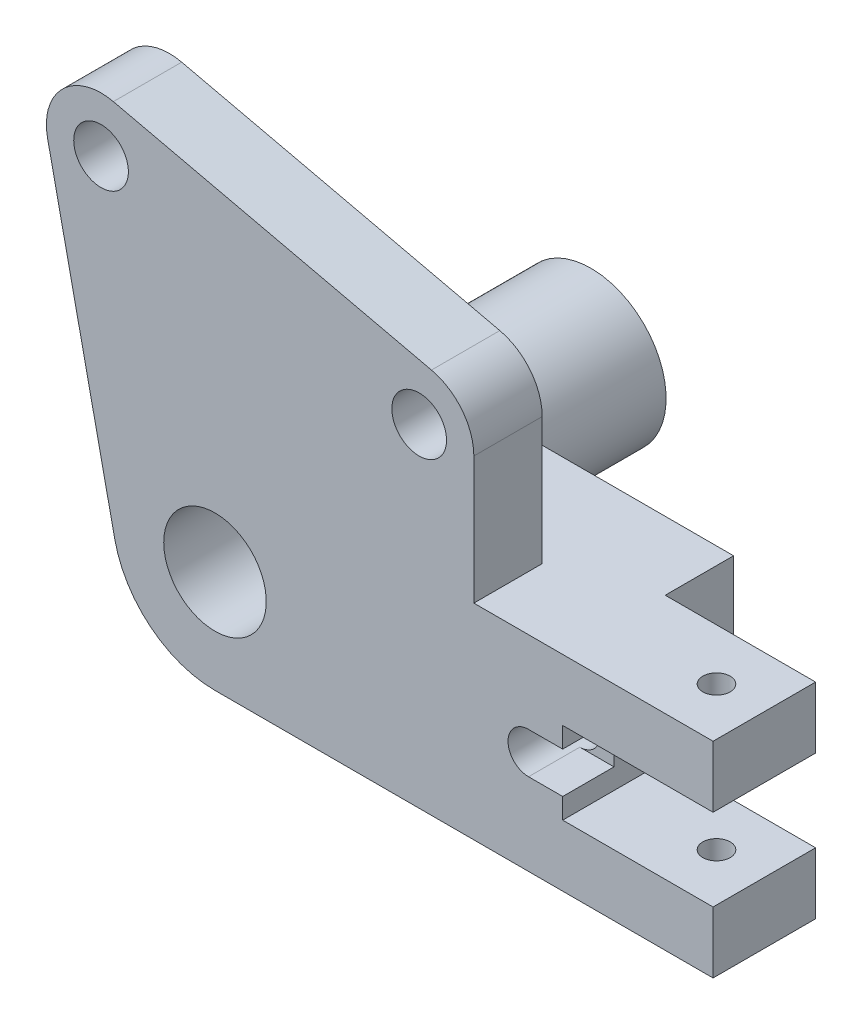
SolidWorks part; units mm, degrees
material "Plain Carbon Steel"
ref_plane "Front Plane" through (0, 0, 0) normal (0, 0, 1) x (1, 0, 0)
ref_plane "Top Plane" through (0, 0, 0) normal (0, 1, 0) x (1, 0, 0)
ref_plane "Right Plane" through (0, 0, 0) normal (1, 0, 0) x (0, 0, -1)
sketch "Bracket Plate Profile" plane through (0, 0, 0) normal (0, 0, 1) x (1, 0, 0)
  line L0 (0, 0) -> (-72.8738, 0)
  line L1 (-87.5408, 11.8571) -> (-97.3643, 57.7001)
  line L2 (-87.743, 67.1715) -> (-41.2011, 56.431)
  line L3 (-35, 48.6359) -> (-35, 30)
  line L4 (-35, 30) -> (0, 30)
  line L5 (0, 30) -> (0, 21)
  line L6 (0, 21) -> (-22, 21)
  line L7 (-22, 21) -> (-22, 9)
  line L8 (-22, 9) -> (0, 9)
  line L9 (0, 9) -> (0, 0)
  arc A0 (-35, 48.6359) -> (-41.2011, 56.431) centre (-43, 48.6359) ccw
  arc A1 (-87.743, 67.1715) -> (-97.3643, 57.7001) centre (-89.5419, 59.3763) ccw
  circle A2 centre (-89.5419, 59.3763) radius 4
  circle A3 centre (-43, 48.6359) radius 4
  arc A4 (-72.8738, 0) -> (-87.5408, 11.8571) centre (-72.8738, 15) cw
  point P13 (-35, 55)
  point P16 (-100, 70)
  point P21 (-85, 0)
  dimension "D9" = 8
  dimension "D10" = 8
  dimension "D11" = 15
  dimension "D1" = 85
  dimension "D2" = 100
  dimension "D3" = 70
  dimension "D4" = 30
  dimension "D5" = 65
  dimension "D6" = 25
  dimension "D7" = 12
  dimension "D8" = 22
extrude "Bracket Plate" add sketch "Bracket Plate Profile" along normal blind 25
sketch "Fork Slot Sketch" plane through (0, 30, 0) normal (0, 1, 0) x (1, 0, 0)
  line L0 (-35, -25) -> (-35, 0) construction
  line L1 (-35, -15) -> (-115.7544, -15)
  line L2 (-35, -15) -> (-35, 6.2579)
  line L3 (-35, 6.2579) -> (-115.7544, 6.2579)
  line L4 (-115.7544, -15) -> (-115.7544, 6.2579)
  line L5 (-41.2011, -25) -> (-87.743, -25) construction
  line L6 (0, 0) -> (-35, 0) construction
  dimension "D1" = 10
  dimension "D2" = 80.7544
  dimension "D3" = 6.2579
extrude "Fork Slot" cut sketch "Fork Slot Sketch" along normal through all
sketch "Pivot Boss Sketch" plane through (0, 0, 0) normal (0, 0, -1) x (-1, 0, 0)
  circle A0 centre (72.8738, 15) radius 11
  arc A1 (72.8738, 0) -> (87.5408, 11.8571) centre (72.8738, 15) ccw construction
  dimension "D1" = 22
extrude "Pivot Boss Ø22" add sketch "Pivot Boss Sketch" along normal blind 30
sketch "Pivot Bore Sketch" plane through (0, 0, -30) normal (0, 0, -1) x (-1, 0, 0)
  circle A0 centre (72.8738, 15) radius 7.5
  dimension "D1" = 15
extrude "Pivot Bore Ø15" cut sketch "Pivot Bore Sketch" against normal through all
sketch "Fork Notch Sketch" plane through (0, 30, 0) normal (0, 1, 0) x (1, 0, 0)
  line L0 (0, -25) -> (0, 0) construction
  line L1 (0, -10) -> (-22, -10)
  line L2 (0, -10) -> (0, 9.4983)
  line L3 (0, 9.4983) -> (-22, 9.4983)
  line L4 (-22, -10) -> (-22, 9.4983)
  line L5 (0, 0) -> (-91.4286, 0) construction
  dimension "D1" = 22
  dimension "D2" = 10
  dimension "D3" = 9.4983
extrude "Fork Notch 22x10" cut sketch "Fork Notch Sketch" against normal through all
sketch "Fork Pin Hole Sketch" plane through (0, 30, 0) normal (0, 1, 0) x (1, 0, 0)
  line L0 (0, -25) -> (0, -10) construction
  circle A0 centre (-7, -17.5) radius 2
  point P5 (0, -17.5)
  dimension "D1" = 7
  dimension "D2" = 4
extrude "Fork Pin Hole" cut sketch "Fork Pin Hole Sketch" against normal blind 30
sketch "Clamp Hole Sketch" plane through (0, 0, 25) normal (0, 0, 1) x (1, 0, 0)
  line L0 (-22, 9) -> (-22, 21) construction
  circle A0 centre (-27, 15) radius 3
  point P5 (-22, 15)
  dimension "D1" = 6
  dimension "D2" = 5
extrude "Clamp Hole" cut sketch "Clamp Hole Sketch" against normal blind 30
sketch "Clamp Pocket Sketch" plane through (0, 0, 25) normal (0, 0, 1) x (1, 0, 0)
  line L0 (-35, 30) -> (-35, 48.6359) construction
  line L1 (-27, 18) -> (-19.7781, 18)
  line L2 (-27, 18) -> (-27, 12)
  line L3 (-27, 12) -> (-19.7781, 12)
  line L4 (-19.7781, 18) -> (-19.7781, 12)
  circle A0 centre (-27, 15) radius 3 construction
  dimension "D1" = 8
  dimension "D2" = 15.2219
extrude "Clamp Pocket 7.5 Deep" cut sketch "Clamp Pocket Sketch" against normal blind 7.5
sketch "Hole Ø12 Sketch" plane through (0, 0, 0) normal (0, 0, -1) x (-1, 0, 0)
  line L0 (22, 0) -> (22, 30) construction
  line L1 (72.8738, 0) -> (22, 0) construction
  circle A1 centre (27, 15) radius 6
  dimension "D1" = 12
  dimension "D2" = 5
  dimension "D3" = 15
extrude "Hole Ø12" cut sketch "Hole Ø12 Sketch" against normal up to surface (10 mm away) up to face at (-11, 25.5, 10)
